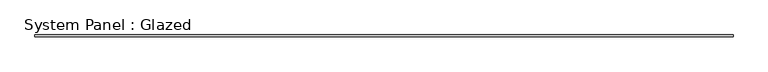
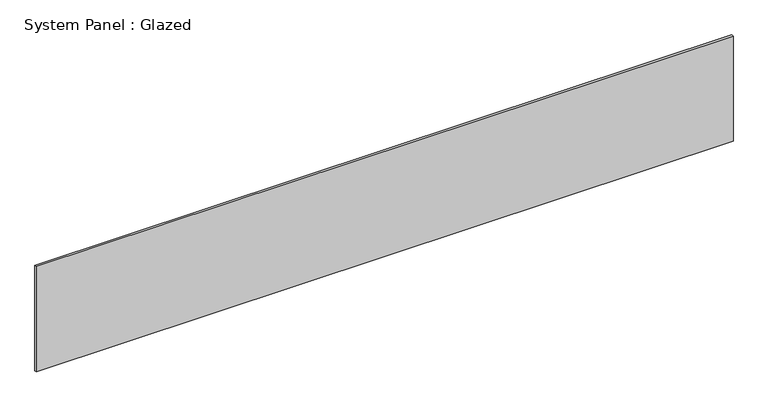
"""IFC4 building model written with IfcOpenShell, lengths in millimetres: plate geometry, System Panel : Glazed."""

from ifc_helpers import new_model, si_unit, origin, origin_with_axes, place, context, project, spatial, polyline, outline, extrude, source, transform, mapped, element, save


def system_panel_glazed_8414a7a5(model_context):
    return source(origin(), model_context, "Body", "SweptSolid", [
        extrude(outline(polyline([(4565.1851423, 19.05), (-4565.1851423, 19.05), (-4565.1851423, 44.45), (4565.1851423, 44.45), (4565.1851423, 19.05)])), origin_with_axes(), (0.0, 0.0, 1.0), 1460.5),
    ])


if __name__ == "__main__":
    model = new_model("IFC4")
    model_context = context("Model", 3, world=origin())
    ifc_project = project(units=[si_unit("LENGTHUNIT", "METRE", prefix="MILLI")], contexts=[model_context])
    site = spatial("IfcSite", under=ifc_project)
    building = spatial("IfcBuilding", under=site)
    placement = place(None, origin())
    system_panel_glazed_shape = system_panel_glazed_8414a7a5(model_context)
    element("IfcPlate", 1, ObjectType="System Panel : Glazed", at=placement, inside=building, context=model_context, shape_type="MappedRepresentation", body=[
        mapped(system_panel_glazed_shape, transform((0.0, 0.0, 0.0), x_axis=(1.0, 0.0, 0.0), y_axis=(0.0, 1.0, 0.0), z_axis=(0.0, 0.0, 1.0))),
    ])
    save(model, "model.ifc")

# Revit data of these elements
# Type "System Panel : Glazed"
#   Construction Type Id = "GSP4R"
#   Analytic Construction = "1/8 in Pilkington single glazing"
#   Visual Light Transmittance = 0.9
#   Solar Heat Gain Coefficient = 0.86
#   Heat Transfer Coefficient (U) = 1.18115 BTU/(h·ft²·°F)
# Element 1 (IfcPlate, "System Panel : Glazed")
#   Materials on its faces: "Glass"
# Materials
#   "Glass": class "Glass", colour RGB 0 128 192, transparency 0.75, Description = "Soda Lime Glass", Cost = 0
